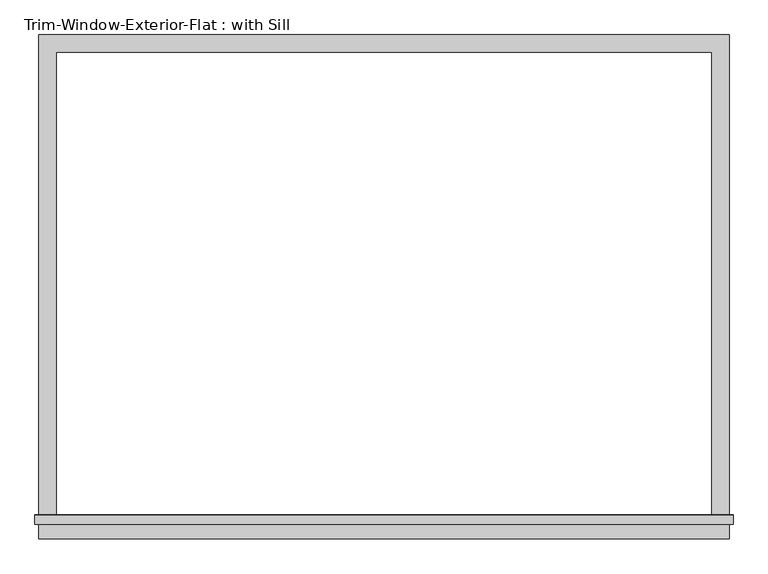
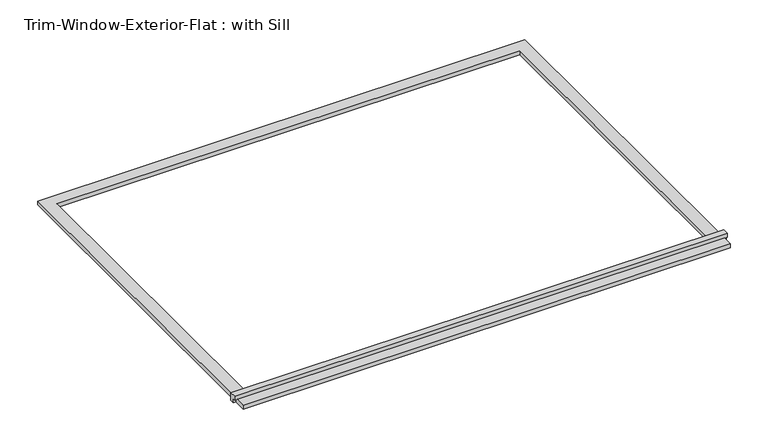
"""IFC4 building model written with IfcOpenShell, lengths in millimetres: proxy geometry, Trim-Window-Exterior-Flat : with Sill."""

from ifc_helpers import new_model, si_unit, frame, origin, origin_with_axes, place, context, project, spatial, polyline, outline, extrude, source, transform, mapped, element, save


def trim_window_exterior_flat_with_sill_088bf4ff(model_context):
    return source(origin(), model_context, "Body", "SweptSolid", [
        extrude(outline(polyline([(1136.65, -1546.1823709), (1136.65, -1603.3323709), (-1136.65, -1603.3323709), (-1136.65, -1546.1823709), (1136.65, -1546.1823709)])), origin_with_axes(), (0.0, 0.0, 1.0), 19.05),
        extrude(outline(polyline([(-1555.75, 38.1), (-1526.4580645, 38.1), (-1524.0, 19.05), (-1524.0, 0.0), (-1546.1823709, 0.0), (-1546.1823709, 19.05), (-1555.75, 19.05), (-1555.75, 38.1)])), frame((-1149.35, 0.0, 0.0), z_axis=(1.0, 0.0, 0.0), x_axis=(0.0, 1.0, 0.0)), (0.0, 0.0, 1.0), 2298.7),
        extrude(outline(polyline([(-1136.65, 57.15), (1136.65, 57.15), (1136.65, -1524.0), (1079.5, -1524.0), (1079.5, 0.0), (-1079.5, 0.0), (-1079.5, -1524.0), (-1136.65, -1524.0), (-1136.65, 57.15)])), origin_with_axes(), (0.0, 0.0, 1.0), 19.05),
    ])


if __name__ == "__main__":
    model = new_model("IFC4")
    model_context = context("Model", 3, world=origin())
    ifc_project = project(units=[si_unit("LENGTHUNIT", "METRE", prefix="MILLI")], contexts=[model_context])
    site = spatial("IfcSite", under=ifc_project)
    building = spatial("IfcBuilding", under=site)
    placement = place(None, origin())
    trim_window_exterior_flat_with_sill_shape = trim_window_exterior_flat_with_sill_088bf4ff(model_context)
    element("IfcBuildingElementProxy", 1, Name="Trim-Window-Exterior-Flat : with Sill", ObjectType="Trim-Window-Exterior-Flat : with Sill", at=placement, inside=building, context=model_context, shape_type="MappedRepresentation", body=[
        mapped(trim_window_exterior_flat_with_sill_shape, transform((0.0, 0.0, 0.0), x_axis=(1.0, 0.0, 0.0), y_axis=(0.0, 1.0, 0.0), z_axis=(0.0, 0.0, 1.0))),
    ])
    save(model, "model.ifc")

# Revit data of these elements
# Type "Trim-Window-Exterior-Flat : with Sill"
#   Trim Width = 0' - 2 1/4"
#   Trim Thickness_Picture Frame = 0' - 1 1/4"
#   Trim Thickness_with Sill = 0' - 0 3/4"
#   Sill Thickness = 0' - 1 1/4"
#   Opening Width [instance default] = 2' - 0"
#   Opening Height [instance default] = 3' - 0"
#   Default Elevation = 4' - 0"
#   Sill = yes
#   Picture Frame = no
#   Trim Material [instance default] = none
# Element 1 (IfcBuildingElementProxy, "Trim-Window-Exterior-Flat : with Sill")
#   Opening Width = 7' - 1"
#   Opening Height = 5' - 0"
#   Trim Material = Clad - White
#   Materials on its faces: "Clad - White"
# Materials
#   "Clad - White": class "Wood", colour RGB 242 242 238, transparency 0, Cost = 0
